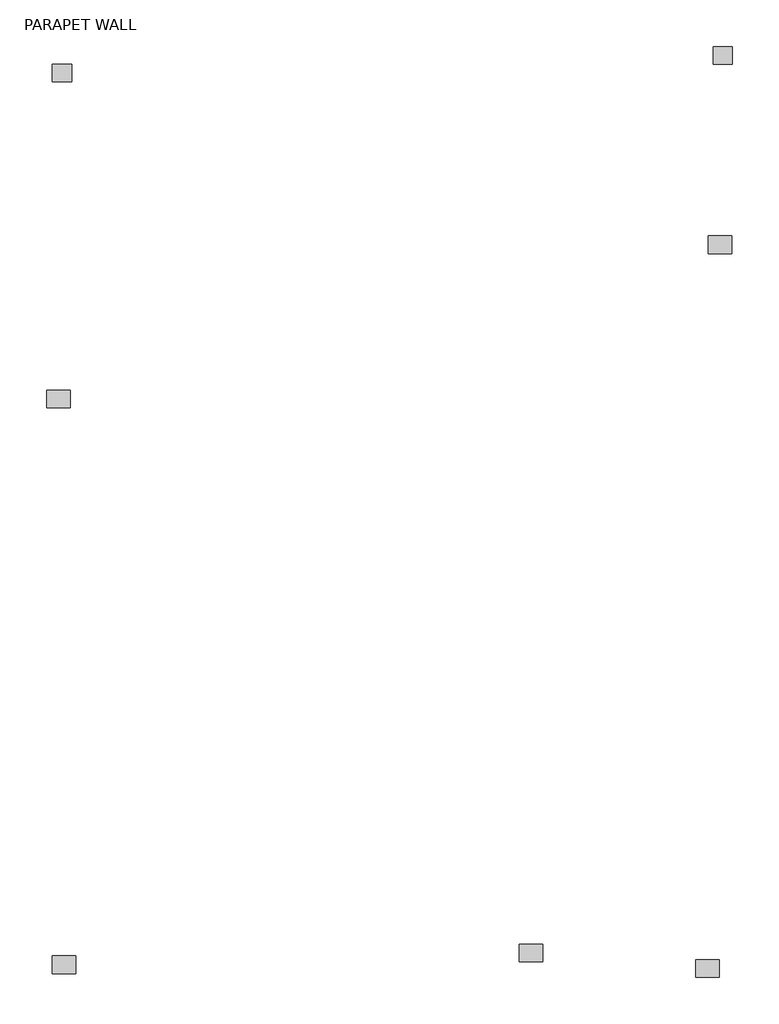
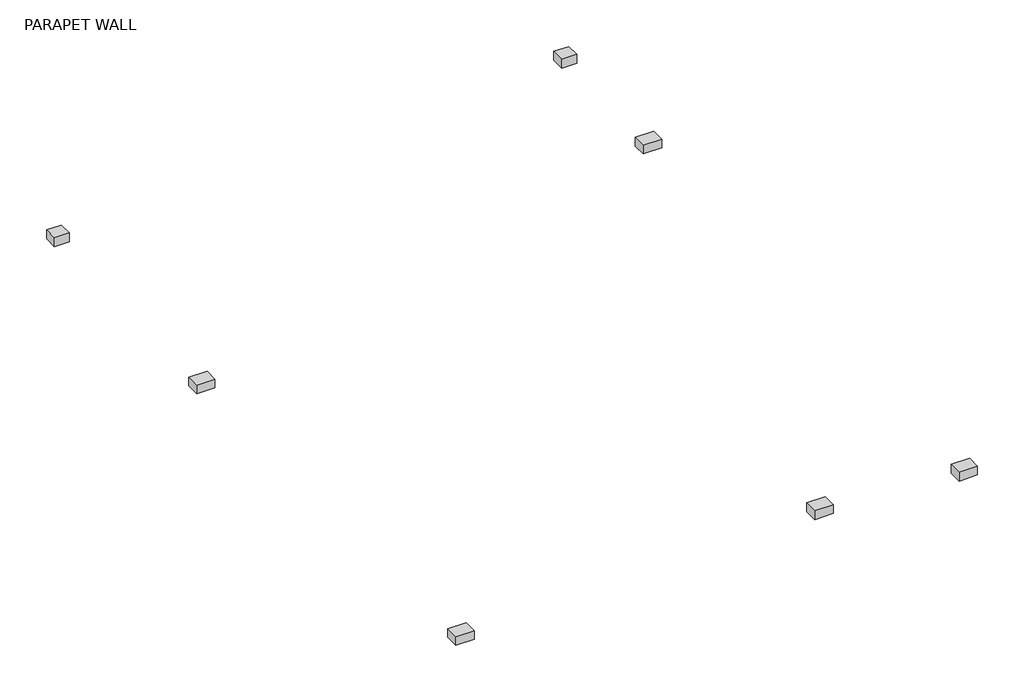
# One storey: 7 columns.
"""IFC4 building model written with IfcOpenShell, lengths in millimetres."""

from ifc_helpers import new_model, si_unit, frame, origin, place, context, project, spatial, polyline, outline, extrude, element, save

model = new_model("IFC4")

# Units and contexts
model_context = context("Model", 3, world=origin())
ifc_project = project(units=[si_unit("LENGTHUNIT", "METRE", prefix="MILLI")], contexts=[model_context])

# Site, building, storey
site = spatial("IfcSite", under=ifc_project)
building = spatial("IfcBuilding", under=site)
storey = spatial("IfcBuildingStorey", under=building, Name="PARAPET WALL", Elevation=8229.6)

# Columns
placement = place(None, origin())
element("IfcColumn", 1, ObjectType="Rectangular Column : 1'9\"", at=placement, inside=storey, context=model_context, shape_type="SweptSolid", body=[
    extrude(outline(polyline([(10828.4334712, 491.3450307), (10828.4334712, 262.7450307), (10523.6334712, 262.7450307), (10523.6334712, 491.3450307), (10828.4334712, 491.3450307)])), frame((0.0, 0.0, 8077.2), z_axis=(0.0, 0.0, 1.0), x_axis=(1.0, 0.0, 0.0)), (0.0, 0.0, 1.0), 152.4),
])
element("IfcColumn", 2, ObjectType="Rectangular Column : 1'9\"", at=placement, inside=storey, context=model_context, shape_type="SweptSolid", body=[
    extrude(outline(polyline([(8542.4334712, 694.5450307), (8542.4334712, 465.9450307), (8237.6334712, 465.9450307), (8237.6334712, 694.5450307), (8542.4334712, 694.5450307)])), frame((0.0, 0.0, 8077.2), z_axis=(0.0, 0.0, 1.0), x_axis=(1.0, 0.0, 0.0)), (0.0, 0.0, 1.0), 152.4),
])
element("IfcColumn", 3, ObjectType="Rectangular Column : 1'9\"", at=placement, inside=storey, context=model_context, shape_type="SweptSolid", body=[
    extrude(outline(polyline([(2484.5334712, 542.1450307), (2484.5334712, 313.5450307), (2179.7334712, 313.5450307), (2179.7334712, 542.1450307), (2484.5334712, 542.1450307)])), frame((0.0, 0.0, 8077.2), z_axis=(0.0, 0.0, 1.0), x_axis=(1.0, 0.0, 0.0)), (0.0, 0.0, 1.0), 152.4),
])
element("IfcColumn", 4, ObjectType="Rectangular Column : 1'9\"", at=placement, inside=storey, context=model_context, shape_type="SweptSolid", body=[
    extrude(outline(polyline([(2408.3334712, 7882.7450307), (2408.3334712, 7654.1450307), (2103.5334712, 7654.1450307), (2103.5334712, 7882.7450307), (2408.3334712, 7882.7450307)])), frame((0.0, 0.0, 8077.2), z_axis=(0.0, 0.0, 1.0), x_axis=(1.0, 0.0, 0.0)), (0.0, 0.0, 1.0), 152.4),
])
element("IfcColumn", 5, ObjectType="Rectangular Column : 1'9\"", at=placement, inside=storey, context=model_context, shape_type="SweptSolid", body=[
    extrude(outline(polyline([(2179.7334712, 11883.2450307), (2179.7334712, 12111.8450307), (2427.3834712, 12111.8450307), (2427.3834712, 11883.2450307), (2179.7334712, 11883.2450307)])), frame((0.0, 0.0, 8077.2), z_axis=(0.0, 0.0, 1.0), x_axis=(1.0, 0.0, 0.0)), (0.0, 0.0, 1.0), 152.4),
])
element("IfcColumn", 6, ObjectType="Rectangular Column : 1'9\"", at=placement, inside=storey, context=model_context, shape_type="SweptSolid", body=[
    extrude(outline(polyline([(10752.2334712, 12111.8450307), (10752.2334712, 12340.4450307), (10999.8834712, 12340.4450307), (10999.8834712, 12111.8450307), (10752.2334712, 12111.8450307)])), frame((0.0, 0.0, 8077.2), z_axis=(0.0, 0.0, 1.0), x_axis=(1.0, 0.0, 0.0)), (0.0, 0.0, 1.0), 152.4),
])
element("IfcColumn", 7, ObjectType="Rectangular Column : 1'9\"", at=placement, inside=storey, context=model_context, shape_type="SweptSolid", body=[
    extrude(outline(polyline([(10993.5334712, 9882.9950307), (10993.5334712, 9654.3950307), (10688.7334712, 9654.3950307), (10688.7334712, 9882.9950307), (10993.5334712, 9882.9950307)])), frame((0.0, 0.0, 8077.2), z_axis=(0.0, 0.0, 1.0), x_axis=(1.0, 0.0, 0.0)), (0.0, 0.0, 1.0), 152.4),
])

save(model, "model.ifc")

# Revit data of these elements
# Type "Rectangular Column : 1'9\""
#   Assembly Code = "B1010200"
#   Depth = 0' - 9"
#   Offset Base = 0' - 0"
#   Offset Top = 0' - 0"
#   Width = 1' - 0"
#   Material = none
# Elements 1, 2, 3, 4, 7 (IfcColumn, "Rectangular Column : 1'9\"")
#   Phase Created = New Construction
# Elements 5, 6 (IfcColumn, "Rectangular Column : 1'9\"")
#   Phase Created = New Construction
#   Materials on its faces: "Default Wall"
# Materials
#   "Default Wall": colour RGB 128 128 128, transparency 0, Cost = 0
